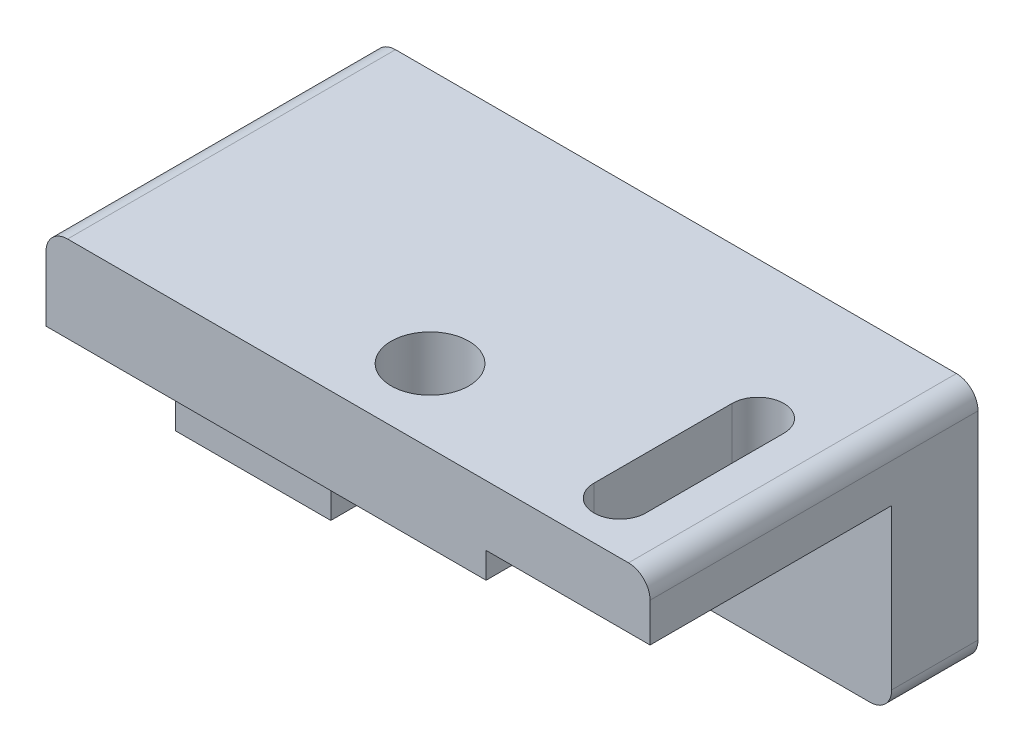
ISO-10303-21;
HEADER;
FILE_DESCRIPTION(('STEP AP214'),'2;1');
FILE_NAME('part.step','',(''),(''),'','','');
FILE_SCHEMA(('AUTOMOTIVE_DESIGN { 1 0 10303 214 1 1 1 1 }'));
ENDSEC;
DATA;
#1=APPLICATION_CONTEXT('core data for automotive mechanical design processes');
#2=APPLICATION_PROTOCOL_DEFINITION('international standard','automotive_design',2000,#1);
#3=PRODUCT_CONTEXT('',#1,'mechanical');
#4=PRODUCT('Part','Part','',(#3));
#5=PRODUCT_RELATED_PRODUCT_CATEGORY('part','',(#4));
#6=PRODUCT_DEFINITION_FORMATION('','',#4);
#7=PRODUCT_DEFINITION_CONTEXT('part definition',#1,'design');
#8=PRODUCT_DEFINITION('design','',#6,#7);
#9=PRODUCT_DEFINITION_SHAPE('','',#8);
#10=(LENGTH_UNIT() NAMED_UNIT(*) SI_UNIT(.MILLI.,.METRE.));
#11=(NAMED_UNIT(*) PLANE_ANGLE_UNIT() SI_UNIT($,.RADIAN.));
#12=(NAMED_UNIT(*) SI_UNIT($,.STERADIAN.) SOLID_ANGLE_UNIT());
#13=UNCERTAINTY_MEASURE_WITH_UNIT(LENGTH_MEASURE(1.E-05),#10,'distance_accuracy_value','');
#14=(GEOMETRIC_REPRESENTATION_CONTEXT(3) GLOBAL_UNCERTAINTY_ASSIGNED_CONTEXT((#13)) GLOBAL_UNIT_ASSIGNED_CONTEXT((#10,
#11,#12)) REPRESENTATION_CONTEXT('',''));
#15=CARTESIAN_POINT('',(0.,0.,0.));
#16=DIRECTION('',(0.,0.,1.));
#17=DIRECTION('',(1.,0.,0.));
#18=AXIS2_PLACEMENT_3D('',#15,#16,#17);
#19=CARTESIAN_POINT('',(0.,-51.,20.));
#20=DIRECTION('',(0.,0.,1.));
#21=DIRECTION('',(0.,-1.,0.));
#22=AXIS2_PLACEMENT_3D('',#19,#20,#21);
#23=PLANE('',#22);
#24=DIRECTION('',(0.,-1.,0.));
#25=VECTOR('',#24,1.);
#26=CARTESIAN_POINT('',(51.,-56.,20.));
#27=LINE('',#26,#25);
#28=CARTESIAN_POINT('',(51.,-34.,20.));
#29=VERTEX_POINT('',#28);
#30=CARTESIAN_POINT('',(51.,-56.,20.));
#31=VERTEX_POINT('',#30);
#32=EDGE_CURVE('E258',#29,#31,#27,.T.);
#33=ORIENTED_EDGE('',*,*,#32,.F.);
#34=DIRECTION('',(-1.,0.,0.));
#35=VECTOR('',#34,1.);
#36=CARTESIAN_POINT('',(51.,-34.,20.));
#37=LINE('',#36,#35);
#38=CARTESIAN_POINT('',(81.,-34.,20.));
#39=VERTEX_POINT('',#38);
#40=EDGE_CURVE('E270',#39,#29,#37,.T.);
#41=ORIENTED_EDGE('',*,*,#40,.F.);
#42=DIRECTION('',(0.,1.,0.));
#43=VECTOR('',#42,1.);
#44=CARTESIAN_POINT('',(81.,-34.,20.));
#45=LINE('',#44,#43);
#46=CARTESIAN_POINT('',(81.,-56.,20.));
#47=VERTEX_POINT('',#46);
#48=EDGE_CURVE('E255',#47,#39,#45,.T.);
#49=ORIENTED_EDGE('',*,*,#48,.F.);
#50=DIRECTION('',(1.,0.,0.));
#51=VECTOR('',#50,1.);
#52=CARTESIAN_POINT('',(36.,-56.,20.));
#53=LINE('',#52,#51);
#54=CARTESIAN_POINT('',(135.,-56.,20.));
#55=VERTEX_POINT('',#54);
#56=EDGE_CURVE('E292',#47,#55,#53,.T.);
#57=ORIENTED_EDGE('',*,*,#56,.T.);
#58=CARTESIAN_POINT('',(135.,-51.,20.));
#59=DIRECTION('',(0.,0.,-1.));
#60=DIRECTION('',(1.,0.,0.));
#61=AXIS2_PLACEMENT_3D('',#58,#59,#60);
#62=CIRCLE('',#61,5.);
#63=CARTESIAN_POINT('',(140.,-51.,20.));
#64=VERTEX_POINT('',#63);
#65=EDGE_CURVE('E283',#64,#55,#62,.T.);
#66=ORIENTED_EDGE('',*,*,#65,.F.);
#67=DIRECTION('',(0.,-1.,0.));
#68=VECTOR('',#67,1.);
#69=CARTESIAN_POINT('',(140.,-51.,20.));
#70=LINE('',#69,#68);
#71=CARTESIAN_POINT('',(140.,-14.,20.));
#72=VERTEX_POINT('',#71);
#73=EDGE_CURVE('E361',#72,#64,#70,.T.);
#74=ORIENTED_EDGE('',*,*,#73,.F.);
#75=DIRECTION('',(-1.,0.,0.));
#76=VECTOR('',#75,1.);
#77=CARTESIAN_POINT('',(140.,-14.,20.));
#78=LINE('',#77,#76);
#79=CARTESIAN_POINT('',(102.,-14.,20.));
#80=VERTEX_POINT('',#79);
#81=EDGE_CURVE('E346',#72,#80,#78,.T.);
#82=ORIENTED_EDGE('',*,*,#81,.T.);
#83=DIRECTION('',(0.,-1.,0.));
#84=VECTOR('',#83,1.);
#85=CARTESIAN_POINT('',(102.,-14.,20.));
#86=LINE('',#85,#84);
#87=CARTESIAN_POINT('',(102.,-20.,20.));
#88=VERTEX_POINT('',#87);
#89=EDGE_CURVE('E352',#80,#88,#86,.T.);
#90=ORIENTED_EDGE('',*,*,#89,.T.);
#91=DIRECTION('',(1.,0.,0.));
#92=VECTOR('',#91,1.);
#93=CARTESIAN_POINT('',(0.,-20.,20.));
#94=LINE('',#93,#92);
#95=CARTESIAN_POINT('',(36.,-20.,20.));
#96=VERTEX_POINT('',#95);
#97=EDGE_CURVE('E369',#96,#88,#94,.T.);
#98=ORIENTED_EDGE('',*,*,#97,.F.);
#99=DIRECTION('',(0.,-1.,0.));
#100=VECTOR('',#99,1.);
#101=CARTESIAN_POINT('',(36.,-20.,20.));
#102=LINE('',#101,#100);
#103=CARTESIAN_POINT('',(36.,-56.,20.));
#104=VERTEX_POINT('',#103);
#105=EDGE_CURVE('E299',#96,#104,#102,.T.);
#106=ORIENTED_EDGE('',*,*,#105,.T.);
#107=EDGE_CURVE('E291',#104,#31,#53,.T.);
#108=ORIENTED_EDGE('',*,*,#107,.T.);
#109=EDGE_LOOP('',(#33,#41,#49,#57,#66,#74,#82,#90,#98,#106,#108));
#110=FACE_BOUND('',#109,.T.);
#111=ADVANCED_FACE('F44',(#110),#23,.T.);
#112=CARTESIAN_POINT('',(140.,-20.,76.));
#113=DIRECTION('',(0.,1.,0.));
#114=DIRECTION('',(0.,0.,1.));
#115=AXIS2_PLACEMENT_3D('',#112,#113,#114);
#116=PLANE('',#115);
#117=CARTESIAN_POINT('',(72.,-20.,59.));
#118=DIRECTION('',(0.,-1.,0.));
#119=DIRECTION('',(0.,0.,-1.));
#120=AXIS2_PLACEMENT_3D('',#117,#118,#119);
#121=CIRCLE('',#120,9.);
#122=CARTESIAN_POINT('',(72.,-20.,50.));
#123=VERTEX_POINT('',#122);
#124=EDGE_CURVE('E276',#123,#123,#121,.T.);
#125=ORIENTED_EDGE('',*,*,#124,.F.);
#126=EDGE_LOOP('',(#125));
#127=FACE_BOUND('',#126,.T.);
#128=DIRECTION('',(0.,0.,-1.));
#129=VECTOR('',#128,1.);
#130=CARTESIAN_POINT('',(0.,-20.,76.));
#131=LINE('',#130,#129);
#132=CARTESIAN_POINT('',(0.,-20.,76.));
#133=VERTEX_POINT('',#132);
#134=CARTESIAN_POINT('',(0.,-20.,46.));
#135=VERTEX_POINT('',#134);
#136=EDGE_CURVE('E388',#133,#135,#131,.T.);
#137=ORIENTED_EDGE('',*,*,#136,.T.);
#138=DIRECTION('',(-1.,0.,0.));
#139=VECTOR('',#138,1.);
#140=CARTESIAN_POINT('',(36.,-20.,46.));
#141=LINE('',#140,#139);
#142=CARTESIAN_POINT('',(36.,-20.,46.));
#143=VERTEX_POINT('',#142);
#144=EDGE_CURVE('E311',#143,#135,#141,.T.);
#145=ORIENTED_EDGE('',*,*,#144,.F.);
#146=DIRECTION('',(0.,0.,-1.));
#147=VECTOR('',#146,1.);
#148=CARTESIAN_POINT('',(36.,-20.,20.));
#149=LINE('',#148,#147);
#150=EDGE_CURVE('E306',#143,#96,#149,.T.);
#151=ORIENTED_EDGE('',*,*,#150,.T.);
#152=ORIENTED_EDGE('',*,*,#97,.T.);
#153=DIRECTION('',(0.,0.,1.));
#154=VECTOR('',#153,1.);
#155=CARTESIAN_POINT('',(102.,-20.,20.));
#156=LINE('',#155,#154);
#157=CARTESIAN_POINT('',(102.,-20.,76.));
#158=VERTEX_POINT('',#157);
#159=EDGE_CURVE('E359',#88,#158,#156,.T.);
#160=ORIENTED_EDGE('',*,*,#159,.T.);
#161=DIRECTION('',(1.,0.,0.));
#162=VECTOR('',#161,1.);
#163=CARTESIAN_POINT('',(140.,-20.,76.));
#164=LINE('',#163,#162);
#165=EDGE_CURVE('E374',#133,#158,#164,.T.);
#166=ORIENTED_EDGE('',*,*,#165,.F.);
#167=EDGE_LOOP('',(#137,#145,#151,#152,#160,#166));
#168=FACE_BOUND('',#167,.T.);
#169=ADVANCED_FACE('F50',(#127,#168),#116,.F.);
#170=CARTESIAN_POINT('',(140.,-5.00000000000004,76.));
#171=DIRECTION('',(-1.,0.,0.));
#172=DIRECTION('',(0.,0.,1.));
#173=AXIS2_PLACEMENT_3D('',#170,#171,#172);
#174=PLANE('',#173);
#175=ORIENTED_EDGE('',*,*,#73,.T.);
#176=DIRECTION('',(0.,0.,1.));
#177=VECTOR('',#176,1.);
#178=CARTESIAN_POINT('',(140.,-51.,-84.));
#179=LINE('',#178,#177);
#180=CARTESIAN_POINT('',(140.,-51.,0.));
#181=VERTEX_POINT('',#180);
#182=EDGE_CURVE('E289',#181,#64,#179,.T.);
#183=ORIENTED_EDGE('',*,*,#182,.F.);
#184=DIRECTION('',(0.,1.,0.));
#185=VECTOR('',#184,1.);
#186=CARTESIAN_POINT('',(140.,-5.00000000000004,0.));
#187=LINE('',#186,#185);
#188=CARTESIAN_POINT('',(140.,-5.00000000000004,0.));
#189=VERTEX_POINT('',#188);
#190=EDGE_CURVE('E372',#181,#189,#187,.T.);
#191=ORIENTED_EDGE('',*,*,#190,.T.);
#192=DIRECTION('',(0.,0.,-1.));
#193=VECTOR('',#192,1.);
#194=CARTESIAN_POINT('',(140.,-5.00000000000004,76.));
#195=LINE('',#194,#193);
#196=CARTESIAN_POINT('',(140.,-5.00000000000004,76.));
#197=VERTEX_POINT('',#196);
#198=EDGE_CURVE('E53',#197,#189,#195,.T.);
#199=ORIENTED_EDGE('',*,*,#198,.F.);
#200=DIRECTION('',(0.,1.,0.));
#201=VECTOR('',#200,1.);
#202=CARTESIAN_POINT('',(140.,-5.00000000000004,76.));
#203=LINE('',#202,#201);
#204=CARTESIAN_POINT('',(140.,-14.,76.));
#205=VERTEX_POINT('',#204);
#206=EDGE_CURVE('E377',#205,#197,#203,.T.);
#207=ORIENTED_EDGE('',*,*,#206,.F.);
#208=DIRECTION('',(0.,0.,1.));
#209=VECTOR('',#208,1.);
#210=CARTESIAN_POINT('',(140.,-14.,20.));
#211=LINE('',#210,#209);
#212=EDGE_CURVE('E358',#72,#205,#211,.T.);
#213=ORIENTED_EDGE('',*,*,#212,.F.);
#214=EDGE_LOOP('',(#175,#183,#191,#199,#207,#213));
#215=FACE_BOUND('',#214,.T.);
#216=ADVANCED_FACE('F439',(#215),#174,.F.);
#217=CARTESIAN_POINT('',(135.,-5.,76.));
#218=DIRECTION('',(0.,0.,-1.));
#219=DIRECTION('',(-1.,0.,0.));
#220=AXIS2_PLACEMENT_3D('',#217,#218,#219);
#221=CYLINDRICAL_SURFACE('',#220,5.);
#222=CARTESIAN_POINT('',(135.,-5.,0.));
#223=DIRECTION('',(0.,0.,1.));
#224=DIRECTION('',(1.,0.,0.));
#225=AXIS2_PLACEMENT_3D('',#222,#223,#224);
#226=CIRCLE('',#225,5.);
#227=CARTESIAN_POINT('',(135.,0.,0.));
#228=VERTEX_POINT('',#227);
#229=EDGE_CURVE('E392',#189,#228,#226,.T.);
#230=ORIENTED_EDGE('',*,*,#229,.T.);
#231=DIRECTION('',(0.,0.,-1.));
#232=VECTOR('',#231,1.);
#233=CARTESIAN_POINT('',(135.,0.,76.));
#234=LINE('',#233,#232);
#235=CARTESIAN_POINT('',(135.,0.,76.));
#236=VERTEX_POINT('',#235);
#237=EDGE_CURVE('E409',#236,#228,#234,.T.);
#238=ORIENTED_EDGE('',*,*,#237,.F.);
#239=CARTESIAN_POINT('',(135.,-5.,76.));
#240=DIRECTION('',(0.,0.,1.));
#241=DIRECTION('',(1.,0.,0.));
#242=AXIS2_PLACEMENT_3D('',#239,#240,#241);
#243=CIRCLE('',#242,5.);
#244=EDGE_CURVE('E382',#197,#236,#243,.T.);
#245=ORIENTED_EDGE('',*,*,#244,.F.);
#246=ORIENTED_EDGE('',*,*,#198,.T.);
#247=EDGE_LOOP('',(#230,#238,#245,#246));
#248=FACE_BOUND('',#247,.T.);
#249=ADVANCED_FACE('F411',(#248),#221,.T.);
#250=CARTESIAN_POINT('',(5.00000000000004,0.,76.));
#251=DIRECTION('',(0.,-1.,0.));
#252=DIRECTION('',(0.,0.,-1.));
#253=AXIS2_PLACEMENT_3D('',#250,#251,#252);
#254=PLANE('',#253);
#255=CARTESIAN_POINT('',(72.,0.,59.));
#256=DIRECTION('',(0.,-1.,0.));
#257=DIRECTION('',(0.,0.,-1.));
#258=AXIS2_PLACEMENT_3D('',#255,#256,#257);
#259=CIRCLE('',#258,9.);
#260=CARTESIAN_POINT('',(72.,0.,50.));
#261=VERTEX_POINT('',#260);
#262=EDGE_CURVE('E47',#261,#261,#259,.T.);
#263=ORIENTED_EDGE('',*,*,#262,.T.);
#264=EDGE_LOOP('',(#263));
#265=FACE_BOUND('',#264,.T.);
#266=DIRECTION('',(0.,0.,1.));
#267=VECTOR('',#266,1.);
#268=CARTESIAN_POINT('',(127.,0.,76.));
#269=LINE('',#268,#267);
#270=CARTESIAN_POINT('',(127.,0.,32.));
#271=VERTEX_POINT('',#270);
#272=CARTESIAN_POINT('',(127.,0.,64.));
#273=VERTEX_POINT('',#272);
#274=EDGE_CURVE('E341',#271,#273,#269,.T.);
#275=ORIENTED_EDGE('',*,*,#274,.T.);
#276=CARTESIAN_POINT('',(121.,0.,64.));
#277=DIRECTION('',(0.,-1.,0.));
#278=DIRECTION('',(0.,0.,-1.));
#279=AXIS2_PLACEMENT_3D('',#276,#277,#278);
#280=CIRCLE('',#279,6.);
#281=CARTESIAN_POINT('',(115.,0.,64.));
#282=VERTEX_POINT('',#281);
#283=EDGE_CURVE('E342',#273,#282,#280,.T.);
#284=ORIENTED_EDGE('',*,*,#283,.T.);
#285=DIRECTION('',(0.,0.,-1.));
#286=VECTOR('',#285,1.);
#287=CARTESIAN_POINT('',(115.,0.,76.));
#288=LINE('',#287,#286);
#289=CARTESIAN_POINT('',(115.,0.,32.));
#290=VERTEX_POINT('',#289);
#291=EDGE_CURVE('E328',#282,#290,#288,.T.);
#292=ORIENTED_EDGE('',*,*,#291,.T.);
#293=CARTESIAN_POINT('',(121.,0.,32.));
#294=DIRECTION('',(0.,-1.,0.));
#295=DIRECTION('',(0.,0.,-1.));
#296=AXIS2_PLACEMENT_3D('',#293,#294,#295);
#297=CIRCLE('',#296,6.);
#298=EDGE_CURVE('E339',#290,#271,#297,.T.);
#299=ORIENTED_EDGE('',*,*,#298,.T.);
#300=EDGE_LOOP('',(#275,#284,#292,#299));
#301=FACE_BOUND('',#300,.T.);
#302=DIRECTION('',(-1.,0.,0.));
#303=VECTOR('',#302,1.);
#304=CARTESIAN_POINT('',(5.00000000000004,0.,0.));
#305=LINE('',#304,#303);
#306=CARTESIAN_POINT('',(5.00000000000004,0.,0.));
#307=VERTEX_POINT('',#306);
#308=EDGE_CURVE('E395',#228,#307,#305,.T.);
#309=ORIENTED_EDGE('',*,*,#308,.T.);
#310=DIRECTION('',(0.,0.,-1.));
#311=VECTOR('',#310,1.);
#312=CARTESIAN_POINT('',(5.00000000000004,0.,76.));
#313=LINE('',#312,#311);
#314=CARTESIAN_POINT('',(5.00000000000004,0.,76.));
#315=VERTEX_POINT('',#314);
#316=EDGE_CURVE('E401',#315,#307,#313,.T.);
#317=ORIENTED_EDGE('',*,*,#316,.F.);
#318=DIRECTION('',(-1.,0.,0.));
#319=VECTOR('',#318,1.);
#320=CARTESIAN_POINT('',(5.00000000000004,0.,76.));
#321=LINE('',#320,#319);
#322=EDGE_CURVE('E384',#236,#315,#321,.T.);
#323=ORIENTED_EDGE('',*,*,#322,.F.);
#324=ORIENTED_EDGE('',*,*,#237,.T.);
#325=EDGE_LOOP('',(#309,#317,#323,#324));
#326=FACE_BOUND('',#325,.T.);
#327=ADVANCED_FACE('F430',(#265,#301,#326),#254,.F.);
#328=CARTESIAN_POINT('',(5.,-5.,76.));
#329=DIRECTION('',(0.,0.,-1.));
#330=DIRECTION('',(-1.,0.,0.));
#331=AXIS2_PLACEMENT_3D('',#328,#329,#330);
#332=CYLINDRICAL_SURFACE('',#331,5.);
#333=CARTESIAN_POINT('',(5.,-5.,0.));
#334=DIRECTION('',(0.,0.,1.));
#335=DIRECTION('',(-1.,0.,0.));
#336=AXIS2_PLACEMENT_3D('',#333,#334,#335);
#337=CIRCLE('',#336,5.);
#338=CARTESIAN_POINT('',(0.,-5.00000000000003,0.));
#339=VERTEX_POINT('',#338);
#340=EDGE_CURVE('E393',#307,#339,#337,.T.);
#341=ORIENTED_EDGE('',*,*,#340,.T.);
#342=DIRECTION('',(0.,0.,-1.));
#343=VECTOR('',#342,1.);
#344=CARTESIAN_POINT('',(0.,-5.00000000000003,76.));
#345=LINE('',#344,#343);
#346=CARTESIAN_POINT('',(0.,-5.00000000000003,76.));
#347=VERTEX_POINT('',#346);
#348=EDGE_CURVE('E400',#347,#339,#345,.T.);
#349=ORIENTED_EDGE('',*,*,#348,.F.);
#350=CARTESIAN_POINT('',(5.,-5.,76.));
#351=DIRECTION('',(0.,0.,1.));
#352=DIRECTION('',(-1.,0.,0.));
#353=AXIS2_PLACEMENT_3D('',#350,#351,#352);
#354=CIRCLE('',#353,5.);
#355=EDGE_CURVE('E383',#315,#347,#354,.T.);
#356=ORIENTED_EDGE('',*,*,#355,.F.);
#357=ORIENTED_EDGE('',*,*,#316,.T.);
#358=EDGE_LOOP('',(#341,#349,#356,#357));
#359=FACE_BOUND('',#358,.T.);
#360=ADVANCED_FACE('F431',(#359),#332,.T.);
#361=CARTESIAN_POINT('',(0.,-20.,76.));
#362=DIRECTION('',(1.,0.,0.));
#363=DIRECTION('',(0.,0.,-1.));
#364=AXIS2_PLACEMENT_3D('',#361,#362,#363);
#365=PLANE('',#364);
#366=DIRECTION('',(0.,1.,0.));
#367=VECTOR('',#366,1.);
#368=CARTESIAN_POINT('',(0.,-29.5,27.));
#369=LINE('',#368,#367);
#370=CARTESIAN_POINT('',(0.,-46.5,27.));
#371=VERTEX_POINT('',#370);
#372=CARTESIAN_POINT('',(0.,-29.5,27.));
#373=VERTEX_POINT('',#372);
#374=EDGE_CURVE('E218',#371,#373,#369,.T.);
#375=ORIENTED_EDGE('',*,*,#374,.T.);
#376=CARTESIAN_POINT('',(0.,-29.5,33.));
#377=DIRECTION('',(1.,0.,0.));
#378=DIRECTION('',(0.,0.,-1.));
#379=AXIS2_PLACEMENT_3D('',#376,#377,#378);
#380=CIRCLE('',#379,6.);
#381=CARTESIAN_POINT('',(0.,-29.5,39.));
#382=VERTEX_POINT('',#381);
#383=EDGE_CURVE('E213',#373,#382,#380,.T.);
#384=ORIENTED_EDGE('',*,*,#383,.T.);
#385=DIRECTION('',(0.,-1.,0.));
#386=VECTOR('',#385,1.);
#387=CARTESIAN_POINT('',(0.,-29.5,39.));
#388=LINE('',#387,#386);
#389=CARTESIAN_POINT('',(0.,-46.5,39.));
#390=VERTEX_POINT('',#389);
#391=EDGE_CURVE('E224',#382,#390,#388,.T.);
#392=ORIENTED_EDGE('',*,*,#391,.T.);
#393=CARTESIAN_POINT('',(0.,-46.5,33.));
#394=DIRECTION('',(1.,0.,0.));
#395=DIRECTION('',(0.,0.,-1.));
#396=AXIS2_PLACEMENT_3D('',#393,#394,#395);
#397=CIRCLE('',#396,6.00000000000001);
#398=EDGE_CURVE('E64',#390,#371,#397,.T.);
#399=ORIENTED_EDGE('',*,*,#398,.T.);
#400=EDGE_LOOP('',(#375,#384,#392,#399));
#401=FACE_BOUND('',#400,.T.);
#402=DIRECTION('',(0.,0.,-1.));
#403=VECTOR('',#402,1.);
#404=CARTESIAN_POINT('',(0.,-56.,5.00000000000004));
#405=LINE('',#404,#403);
#406=CARTESIAN_POINT('',(0.,-56.,46.));
#407=VERTEX_POINT('',#406);
#408=CARTESIAN_POINT('',(0.,-56.,0.));
#409=VERTEX_POINT('',#408);
#410=EDGE_CURVE('E370',#407,#409,#405,.T.);
#411=ORIENTED_EDGE('',*,*,#410,.F.);
#412=DIRECTION('',(0.,1.,0.));
#413=VECTOR('',#412,1.);
#414=CARTESIAN_POINT('',(0.,-20.,46.));
#415=LINE('',#414,#413);
#416=EDGE_CURVE('E296',#407,#135,#415,.T.);
#417=ORIENTED_EDGE('',*,*,#416,.T.);
#418=ORIENTED_EDGE('',*,*,#136,.F.);
#419=DIRECTION('',(0.,-1.,0.));
#420=VECTOR('',#419,1.);
#421=CARTESIAN_POINT('',(0.,-20.,76.));
#422=LINE('',#421,#420);
#423=EDGE_CURVE('E386',#347,#133,#422,.T.);
#424=ORIENTED_EDGE('',*,*,#423,.F.);
#425=ORIENTED_EDGE('',*,*,#348,.T.);
#426=DIRECTION('',(0.,-1.,0.));
#427=VECTOR('',#426,1.);
#428=CARTESIAN_POINT('',(0.,-20.,0.));
#429=LINE('',#428,#427);
#430=EDGE_CURVE('E378',#339,#409,#429,.T.);
#431=ORIENTED_EDGE('',*,*,#430,.T.);
#432=EDGE_LOOP('',(#411,#417,#418,#424,#425,#431));
#433=FACE_BOUND('',#432,.T.);
#434=ADVANCED_FACE('F227',(#401,#433),#365,.F.);
#435=CARTESIAN_POINT('',(5.,-5.,76.));
#436=DIRECTION('',(0.,0.,-1.));
#437=DIRECTION('',(-1.,0.,0.));
#438=AXIS2_PLACEMENT_3D('',#435,#436,#437);
#439=PLANE('',#438);
#440=ORIENTED_EDGE('',*,*,#165,.T.);
#441=DIRECTION('',(0.,-1.,0.));
#442=VECTOR('',#441,1.);
#443=CARTESIAN_POINT('',(102.,-14.,76.));
#444=LINE('',#443,#442);
#445=CARTESIAN_POINT('',(102.,-14.,76.));
#446=VERTEX_POINT('',#445);
#447=EDGE_CURVE('E354',#446,#158,#444,.T.);
#448=ORIENTED_EDGE('',*,*,#447,.F.);
#449=DIRECTION('',(-1.,0.,0.));
#450=VECTOR('',#449,1.);
#451=CARTESIAN_POINT('',(140.,-14.,76.));
#452=LINE('',#451,#450);
#453=EDGE_CURVE('E350',#205,#446,#452,.T.);
#454=ORIENTED_EDGE('',*,*,#453,.F.);
#455=ORIENTED_EDGE('',*,*,#206,.T.);
#456=ORIENTED_EDGE('',*,*,#244,.T.);
#457=ORIENTED_EDGE('',*,*,#322,.T.);
#458=ORIENTED_EDGE('',*,*,#355,.T.);
#459=ORIENTED_EDGE('',*,*,#423,.T.);
#460=EDGE_LOOP('',(#440,#448,#454,#455,#456,#457,#458,#459));
#461=FACE_BOUND('',#460,.T.);
#462=ADVANCED_FACE('F434',(#461),#439,.F.);
#463=CARTESIAN_POINT('',(5.,-5.,0.));
#464=DIRECTION('',(0.,0.,-1.));
#465=DIRECTION('',(-1.,0.,0.));
#466=AXIS2_PLACEMENT_3D('',#463,#464,#465);
#467=PLANE('',#466);
#468=CARTESIAN_POINT('',(66.,-45.,0.));
#469=DIRECTION('',(0.,0.,1.));
#470=DIRECTION('',(1.,0.,0.));
#471=AXIS2_PLACEMENT_3D('',#468,#469,#470);
#472=CIRCLE('',#471,6.);
#473=CARTESIAN_POINT('',(72.,-45.,0.));
#474=VERTEX_POINT('',#473);
#475=EDGE_CURVE('E248',#474,#474,#472,.T.);
#476=ORIENTED_EDGE('',*,*,#475,.T.);
#477=EDGE_LOOP('',(#476));
#478=FACE_BOUND('',#477,.T.);
#479=CARTESIAN_POINT('',(135.,-51.,0.));
#480=DIRECTION('',(0.,0.,-1.));
#481=DIRECTION('',(-1.,0.,0.));
#482=AXIS2_PLACEMENT_3D('',#479,#480,#481);
#483=CIRCLE('',#482,5.);
#484=CARTESIAN_POINT('',(135.,-56.,0.));
#485=VERTEX_POINT('',#484);
#486=EDGE_CURVE('E290',#485,#181,#483,.F.);
#487=ORIENTED_EDGE('',*,*,#486,.F.);
#488=DIRECTION('',(-1.,0.,0.));
#489=VECTOR('',#488,1.);
#490=CARTESIAN_POINT('',(140.,-56.,0.));
#491=LINE('',#490,#489);
#492=EDGE_CURVE('E298',#485,#409,#491,.T.);
#493=ORIENTED_EDGE('',*,*,#492,.T.);
#494=ORIENTED_EDGE('',*,*,#430,.F.);
#495=ORIENTED_EDGE('',*,*,#340,.F.);
#496=ORIENTED_EDGE('',*,*,#308,.F.);
#497=ORIENTED_EDGE('',*,*,#229,.F.);
#498=ORIENTED_EDGE('',*,*,#190,.F.);
#499=EDGE_LOOP('',(#487,#493,#494,#495,#496,#497,#498));
#500=FACE_BOUND('',#499,.T.);
#501=ADVANCED_FACE('F422',(#478,#500),#467,.T.);
#502=CARTESIAN_POINT('',(0.,-56.,5.00000000000004));
#503=DIRECTION('',(0.,-1.,0.));
#504=DIRECTION('',(0.,0.,-1.));
#505=AXIS2_PLACEMENT_3D('',#502,#503,#504);
#506=PLANE('',#505);
#507=DIRECTION('',(0.,0.,1.));
#508=VECTOR('',#507,1.);
#509=CARTESIAN_POINT('',(51.,-56.,10.));
#510=LINE('',#509,#508);
#511=CARTESIAN_POINT('',(51.,-56.,10.));
#512=VERTEX_POINT('',#511);
#513=EDGE_CURVE('E274',#512,#31,#510,.T.);
#514=ORIENTED_EDGE('',*,*,#513,.T.);
#515=ORIENTED_EDGE('',*,*,#107,.F.);
#516=DIRECTION('',(0.,0.,1.));
#517=VECTOR('',#516,1.);
#518=CARTESIAN_POINT('',(36.,-56.,46.));
#519=LINE('',#518,#517);
#520=CARTESIAN_POINT('',(36.,-56.,46.));
#521=VERTEX_POINT('',#520);
#522=EDGE_CURVE('E301',#104,#521,#519,.T.);
#523=ORIENTED_EDGE('',*,*,#522,.T.);
#524=DIRECTION('',(-1.,0.,0.));
#525=VECTOR('',#524,1.);
#526=CARTESIAN_POINT('',(36.,-56.,46.));
#527=LINE('',#526,#525);
#528=EDGE_CURVE('E308',#521,#407,#527,.T.);
#529=ORIENTED_EDGE('',*,*,#528,.T.);
#530=ORIENTED_EDGE('',*,*,#410,.T.);
#531=ORIENTED_EDGE('',*,*,#492,.F.);
#532=DIRECTION('',(0.,0.,1.));
#533=VECTOR('',#532,1.);
#534=CARTESIAN_POINT('',(135.,-56.,-84.));
#535=LINE('',#534,#533);
#536=EDGE_CURVE('E11',#55,#485,#535,.F.);
#537=ORIENTED_EDGE('',*,*,#536,.F.);
#538=ORIENTED_EDGE('',*,*,#56,.F.);
#539=DIRECTION('',(0.,0.,1.));
#540=VECTOR('',#539,1.);
#541=CARTESIAN_POINT('',(81.,-56.,10.));
#542=LINE('',#541,#540);
#543=CARTESIAN_POINT('',(81.,-56.,10.));
#544=VERTEX_POINT('',#543);
#545=EDGE_CURVE('E267',#544,#47,#542,.T.);
#546=ORIENTED_EDGE('',*,*,#545,.F.);
#547=DIRECTION('',(1.,0.,0.));
#548=VECTOR('',#547,1.);
#549=CARTESIAN_POINT('',(81.,-56.,10.));
#550=LINE('',#549,#548);
#551=EDGE_CURVE('E253',#512,#544,#550,.T.);
#552=ORIENTED_EDGE('',*,*,#551,.F.);
#553=EDGE_LOOP('',(#514,#515,#523,#529,#530,#531,#537,#538,#546,#552));
#554=FACE_BOUND('',#553,.T.);
#555=ADVANCED_FACE('F463',(#554),#506,.T.);
#556=CARTESIAN_POINT('',(102.,-14.,20.));
#557=DIRECTION('',(-1.,0.,0.));
#558=DIRECTION('',(0.,0.,1.));
#559=AXIS2_PLACEMENT_3D('',#556,#557,#558);
#560=PLANE('',#559);
#561=ORIENTED_EDGE('',*,*,#447,.T.);
#562=ORIENTED_EDGE('',*,*,#159,.F.);
#563=ORIENTED_EDGE('',*,*,#89,.F.);
#564=DIRECTION('',(0.,0.,1.));
#565=VECTOR('',#564,1.);
#566=CARTESIAN_POINT('',(102.,-14.,20.));
#567=LINE('',#566,#565);
#568=EDGE_CURVE('E364',#80,#446,#567,.T.);
#569=ORIENTED_EDGE('',*,*,#568,.T.);
#570=EDGE_LOOP('',(#561,#562,#563,#569));
#571=FACE_BOUND('',#570,.T.);
#572=ADVANCED_FACE('F451',(#571),#560,.F.);
#573=CARTESIAN_POINT('',(140.,-14.,20.));
#574=DIRECTION('',(0.,1.,0.));
#575=DIRECTION('',(0.,0.,1.));
#576=AXIS2_PLACEMENT_3D('',#573,#574,#575);
#577=PLANE('',#576);
#578=DIRECTION('',(0.,0.,-1.));
#579=VECTOR('',#578,1.);
#580=CARTESIAN_POINT('',(115.,-14.,64.));
#581=LINE('',#580,#579);
#582=CARTESIAN_POINT('',(115.,-14.,64.));
#583=VERTEX_POINT('',#582);
#584=CARTESIAN_POINT('',(115.,-14.,32.));
#585=VERTEX_POINT('',#584);
#586=EDGE_CURVE('E319',#583,#585,#581,.T.);
#587=ORIENTED_EDGE('',*,*,#586,.F.);
#588=CARTESIAN_POINT('',(121.,-14.,64.));
#589=DIRECTION('',(0.,-1.,0.));
#590=DIRECTION('',(0.,0.,-1.));
#591=AXIS2_PLACEMENT_3D('',#588,#589,#590);
#592=CIRCLE('',#591,6.);
#593=CARTESIAN_POINT('',(127.,-14.,64.));
#594=VERTEX_POINT('',#593);
#595=EDGE_CURVE('E313',#594,#583,#592,.T.);
#596=ORIENTED_EDGE('',*,*,#595,.F.);
#597=DIRECTION('',(0.,0.,1.));
#598=VECTOR('',#597,1.);
#599=CARTESIAN_POINT('',(127.,-14.,64.));
#600=LINE('',#599,#598);
#601=CARTESIAN_POINT('',(127.,-14.,32.));
#602=VERTEX_POINT('',#601);
#603=EDGE_CURVE('E323',#602,#594,#600,.T.);
#604=ORIENTED_EDGE('',*,*,#603,.F.);
#605=CARTESIAN_POINT('',(121.,-14.,32.));
#606=DIRECTION('',(0.,-1.,0.));
#607=DIRECTION('',(0.,0.,-1.));
#608=AXIS2_PLACEMENT_3D('',#605,#606,#607);
#609=CIRCLE('',#608,6.);
#610=EDGE_CURVE('E324',#585,#602,#609,.T.);
#611=ORIENTED_EDGE('',*,*,#610,.F.);
#612=EDGE_LOOP('',(#587,#596,#604,#611));
#613=FACE_BOUND('',#612,.T.);
#614=ORIENTED_EDGE('',*,*,#453,.T.);
#615=ORIENTED_EDGE('',*,*,#568,.F.);
#616=ORIENTED_EDGE('',*,*,#81,.F.);
#617=ORIENTED_EDGE('',*,*,#212,.T.);
#618=EDGE_LOOP('',(#614,#615,#616,#617));
#619=FACE_BOUND('',#618,.T.);
#620=ADVANCED_FACE('F443',(#613,#619),#577,.F.);
#621=CARTESIAN_POINT('',(121.,42.,64.));
#622=DIRECTION('',(0.,-1.,0.));
#623=DIRECTION('',(0.,0.,-1.));
#624=AXIS2_PLACEMENT_3D('',#621,#622,#623);
#625=CYLINDRICAL_SURFACE('',#624,6.);
#626=DIRECTION('',(0.,-1.,0.));
#627=VECTOR('',#626,1.);
#628=CARTESIAN_POINT('',(127.,42.,64.));
#629=LINE('',#628,#627);
#630=EDGE_CURVE('E330',#273,#594,#629,.T.);
#631=ORIENTED_EDGE('',*,*,#630,.T.);
#632=ORIENTED_EDGE('',*,*,#595,.T.);
#633=DIRECTION('',(0.,-1.,0.));
#634=VECTOR('',#633,1.);
#635=CARTESIAN_POINT('',(115.,42.,64.));
#636=LINE('',#635,#634);
#637=EDGE_CURVE('E329',#282,#583,#636,.T.);
#638=ORIENTED_EDGE('',*,*,#637,.F.);
#639=ORIENTED_EDGE('',*,*,#283,.F.);
#640=EDGE_LOOP('',(#631,#632,#638,#639));
#641=FACE_BOUND('',#640,.T.);
#642=ADVANCED_FACE('F555',(#641),#625,.F.);
#643=CARTESIAN_POINT('',(127.,42.,64.));
#644=DIRECTION('',(1.,0.,0.));
#645=DIRECTION('',(0.,0.,-1.));
#646=AXIS2_PLACEMENT_3D('',#643,#644,#645);
#647=PLANE('',#646);
#648=DIRECTION('',(0.,-1.,0.));
#649=VECTOR('',#648,1.);
#650=CARTESIAN_POINT('',(127.,42.,32.));
#651=LINE('',#650,#649);
#652=EDGE_CURVE('E331',#271,#602,#651,.T.);
#653=ORIENTED_EDGE('',*,*,#652,.T.);
#654=ORIENTED_EDGE('',*,*,#603,.T.);
#655=ORIENTED_EDGE('',*,*,#630,.F.);
#656=ORIENTED_EDGE('',*,*,#274,.F.);
#657=EDGE_LOOP('',(#653,#654,#655,#656));
#658=FACE_BOUND('',#657,.T.);
#659=ADVANCED_FACE('F560',(#658),#647,.F.);
#660=CARTESIAN_POINT('',(121.,42.,32.));
#661=DIRECTION('',(0.,-1.,0.));
#662=DIRECTION('',(0.,0.,-1.));
#663=AXIS2_PLACEMENT_3D('',#660,#661,#662);
#664=CYLINDRICAL_SURFACE('',#663,6.);
#665=DIRECTION('',(0.,-1.,0.));
#666=VECTOR('',#665,1.);
#667=CARTESIAN_POINT('',(115.,42.,32.));
#668=LINE('',#667,#666);
#669=EDGE_CURVE('E334',#290,#585,#668,.T.);
#670=ORIENTED_EDGE('',*,*,#669,.T.);
#671=ORIENTED_EDGE('',*,*,#610,.T.);
#672=ORIENTED_EDGE('',*,*,#652,.F.);
#673=ORIENTED_EDGE('',*,*,#298,.F.);
#674=EDGE_LOOP('',(#670,#671,#672,#673));
#675=FACE_BOUND('',#674,.T.);
#676=ADVANCED_FACE('F564',(#675),#664,.F.);
#677=CARTESIAN_POINT('',(115.,42.,64.));
#678=DIRECTION('',(-1.,0.,0.));
#679=DIRECTION('',(0.,0.,1.));
#680=AXIS2_PLACEMENT_3D('',#677,#678,#679);
#681=PLANE('',#680);
#682=ORIENTED_EDGE('',*,*,#637,.T.);
#683=ORIENTED_EDGE('',*,*,#586,.T.);
#684=ORIENTED_EDGE('',*,*,#669,.F.);
#685=ORIENTED_EDGE('',*,*,#291,.F.);
#686=EDGE_LOOP('',(#682,#683,#684,#685));
#687=FACE_BOUND('',#686,.T.);
#688=ADVANCED_FACE('F572',(#687),#681,.F.);
#689=CARTESIAN_POINT('',(36.,-20.,46.));
#690=DIRECTION('',(0.,0.,1.));
#691=DIRECTION('',(1.,0.,0.));
#692=AXIS2_PLACEMENT_3D('',#689,#690,#691);
#693=PLANE('',#692);
#694=ORIENTED_EDGE('',*,*,#416,.F.);
#695=ORIENTED_EDGE('',*,*,#528,.F.);
#696=DIRECTION('',(0.,1.,0.));
#697=VECTOR('',#696,1.);
#698=CARTESIAN_POINT('',(36.,-20.,46.));
#699=LINE('',#698,#697);
#700=EDGE_CURVE('E303',#521,#143,#699,.T.);
#701=ORIENTED_EDGE('',*,*,#700,.T.);
#702=ORIENTED_EDGE('',*,*,#144,.T.);
#703=EDGE_LOOP('',(#694,#695,#701,#702));
#704=FACE_BOUND('',#703,.T.);
#705=ADVANCED_FACE('F470',(#704),#693,.T.);
#706=CARTESIAN_POINT('',(36.,-51.,15.));
#707=DIRECTION('',(-1.,0.,0.));
#708=DIRECTION('',(0.,0.,1.));
#709=AXIS2_PLACEMENT_3D('',#706,#707,#708);
#710=PLANE('',#709);
#711=DIRECTION('',(0.,-1.,0.));
#712=VECTOR('',#711,1.);
#713=CARTESIAN_POINT('',(36.,-29.5,39.));
#714=LINE('',#713,#712);
#715=CARTESIAN_POINT('',(36.,-29.5,39.));
#716=VERTEX_POINT('',#715);
#717=CARTESIAN_POINT('',(36.,-46.5,39.));
#718=VERTEX_POINT('',#717);
#719=EDGE_CURVE('E237',#716,#718,#714,.T.);
#720=ORIENTED_EDGE('',*,*,#719,.F.);
#721=CARTESIAN_POINT('',(36.,-29.5,33.));
#722=DIRECTION('',(1.,0.,0.));
#723=DIRECTION('',(0.,0.,-1.));
#724=AXIS2_PLACEMENT_3D('',#721,#722,#723);
#725=CIRCLE('',#724,6.);
#726=CARTESIAN_POINT('',(36.,-29.5,27.));
#727=VERTEX_POINT('',#726);
#728=EDGE_CURVE('E66',#727,#716,#725,.T.);
#729=ORIENTED_EDGE('',*,*,#728,.F.);
#730=DIRECTION('',(0.,1.,0.));
#731=VECTOR('',#730,1.);
#732=CARTESIAN_POINT('',(36.,-29.5,27.));
#733=LINE('',#732,#731);
#734=CARTESIAN_POINT('',(36.,-46.5,27.));
#735=VERTEX_POINT('',#734);
#736=EDGE_CURVE('E229',#735,#727,#733,.T.);
#737=ORIENTED_EDGE('',*,*,#736,.F.);
#738=CARTESIAN_POINT('',(36.,-46.5,33.));
#739=DIRECTION('',(1.,0.,0.));
#740=DIRECTION('',(0.,0.,-1.));
#741=AXIS2_PLACEMENT_3D('',#738,#739,#740);
#742=CIRCLE('',#741,6.00000000000001);
#743=EDGE_CURVE('E231',#718,#735,#742,.T.);
#744=ORIENTED_EDGE('',*,*,#743,.F.);
#745=EDGE_LOOP('',(#720,#729,#737,#744));
#746=FACE_BOUND('',#745,.T.);
#747=ORIENTED_EDGE('',*,*,#522,.F.);
#748=ORIENTED_EDGE('',*,*,#105,.F.);
#749=ORIENTED_EDGE('',*,*,#150,.F.);
#750=ORIENTED_EDGE('',*,*,#700,.F.);
#751=EDGE_LOOP('',(#747,#748,#749,#750));
#752=FACE_BOUND('',#751,.T.);
#753=ADVANCED_FACE('F458',(#746,#752),#710,.F.);
#754=CARTESIAN_POINT('',(135.,-51.,-84.));
#755=DIRECTION('',(0.,0.,1.));
#756=DIRECTION('',(1.,0.,0.));
#757=AXIS2_PLACEMENT_3D('',#754,#755,#756);
#758=CYLINDRICAL_SURFACE('',#757,5.);
#759=ORIENTED_EDGE('',*,*,#486,.T.);
#760=ORIENTED_EDGE('',*,*,#182,.T.);
#761=ORIENTED_EDGE('',*,*,#65,.T.);
#762=ORIENTED_EDGE('',*,*,#536,.T.);
#763=EDGE_LOOP('',(#759,#760,#761,#762));
#764=FACE_BOUND('',#763,.T.);
#765=ADVANCED_FACE('F471',(#764),#758,.T.);
#766=CARTESIAN_POINT('',(72.,84.,59.));
#767=DIRECTION('',(0.,-1.,0.));
#768=DIRECTION('',(0.,0.,-1.));
#769=AXIS2_PLACEMENT_3D('',#766,#767,#768);
#770=CYLINDRICAL_SURFACE('',#769,9.);
#771=CARTESIAN_POINT('',(72.,-20.,50.));
#772=CARTESIAN_POINT('',(72.,-19.7916666666667,50.));
#773=CARTESIAN_POINT('',(72.,-19.5833333333333,50.));
#774=CARTESIAN_POINT('',(72.,-19.1666666666667,50.));
#775=CARTESIAN_POINT('',(72.,-18.9583333333333,50.));
#776=CARTESIAN_POINT('',(72.,-18.5416666666667,50.));
#777=CARTESIAN_POINT('',(72.,-18.3333333333333,50.));
#778=CARTESIAN_POINT('',(72.,-17.9166666666667,50.));
#779=CARTESIAN_POINT('',(72.,-17.7083333333333,50.));
#780=CARTESIAN_POINT('',(72.,-17.2916666666667,50.));
#781=CARTESIAN_POINT('',(72.,-17.0833333333333,50.));
#782=CARTESIAN_POINT('',(72.,-16.6666666666667,50.));
#783=CARTESIAN_POINT('',(72.,-16.4583333333333,50.));
#784=CARTESIAN_POINT('',(72.,-16.0416666666667,50.));
#785=CARTESIAN_POINT('',(72.,-15.8333333333333,50.));
#786=CARTESIAN_POINT('',(72.,-15.4166666666667,50.));
#787=CARTESIAN_POINT('',(72.,-15.2083333333333,50.));
#788=CARTESIAN_POINT('',(72.,-14.7916666666667,50.));
#789=CARTESIAN_POINT('',(72.,-14.5833333333333,50.));
#790=CARTESIAN_POINT('',(72.,-14.1666666666667,50.));
#791=CARTESIAN_POINT('',(72.,-13.9583333333333,50.));
#792=CARTESIAN_POINT('',(72.,-13.5416666666667,50.));
#793=CARTESIAN_POINT('',(72.,-13.3333333333333,50.));
#794=CARTESIAN_POINT('',(72.,-12.9166666666667,50.));
#795=CARTESIAN_POINT('',(72.,-12.7083333333333,50.));
#796=CARTESIAN_POINT('',(72.,-12.2916666666667,50.));
#797=CARTESIAN_POINT('',(72.,-12.0833333333333,50.));
#798=CARTESIAN_POINT('',(72.,-11.6666666666667,50.));
#799=CARTESIAN_POINT('',(72.,-11.4583333333333,50.));
#800=CARTESIAN_POINT('',(72.,-11.0416666666667,50.));
#801=CARTESIAN_POINT('',(72.,-10.8333333333333,50.));
#802=CARTESIAN_POINT('',(72.,-10.4166666666667,50.));
#803=CARTESIAN_POINT('',(72.,-10.2083333333333,50.));
#804=CARTESIAN_POINT('',(72.,-9.79166666666666,50.));
#805=CARTESIAN_POINT('',(72.,-9.58333333333333,50.));
#806=CARTESIAN_POINT('',(72.,-9.16666666666666,50.));
#807=CARTESIAN_POINT('',(72.,-8.95833333333333,50.));
#808=CARTESIAN_POINT('',(72.,-8.54166666666666,50.));
#809=CARTESIAN_POINT('',(72.,-8.33333333333333,50.));
#810=CARTESIAN_POINT('',(72.,-7.91666666666666,50.));
#811=CARTESIAN_POINT('',(72.,-7.70833333333333,50.));
#812=CARTESIAN_POINT('',(72.,-7.29166666666666,50.));
#813=CARTESIAN_POINT('',(72.,-7.08333333333333,50.));
#814=CARTESIAN_POINT('',(72.,-6.66666666666666,50.));
#815=CARTESIAN_POINT('',(72.,-6.45833333333333,50.));
#816=CARTESIAN_POINT('',(72.,-6.04166666666666,50.));
#817=CARTESIAN_POINT('',(72.,-5.83333333333333,50.));
#818=CARTESIAN_POINT('',(72.,-5.41666666666666,50.));
#819=CARTESIAN_POINT('',(72.,-5.20833333333332,50.));
#820=CARTESIAN_POINT('',(72.,-4.79166666666666,50.));
#821=CARTESIAN_POINT('',(72.,-4.58333333333332,50.));
#822=CARTESIAN_POINT('',(72.,-4.16666666666666,50.));
#823=CARTESIAN_POINT('',(72.,-3.95833333333332,50.));
#824=CARTESIAN_POINT('',(72.,-3.54166666666666,50.));
#825=CARTESIAN_POINT('',(72.,-3.33333333333332,50.));
#826=CARTESIAN_POINT('',(72.,-2.91666666666666,50.));
#827=CARTESIAN_POINT('',(72.,-2.70833333333332,50.));
#828=CARTESIAN_POINT('',(72.,-2.29166666666665,50.));
#829=CARTESIAN_POINT('',(72.,-2.08333333333332,50.));
#830=CARTESIAN_POINT('',(72.,-1.66666666666665,50.));
#831=CARTESIAN_POINT('',(72.,-1.45833333333332,50.));
#832=CARTESIAN_POINT('',(72.,-1.04166666666665,50.));
#833=CARTESIAN_POINT('',(72.,-0.83333333333332,50.));
#834=CARTESIAN_POINT('',(72.,-0.416666666666653,50.));
#835=CARTESIAN_POINT('',(72.,-0.20833333333332,50.));
#836=CARTESIAN_POINT('',(72.,0.,50.));
#837=B_SPLINE_CURVE_WITH_KNOTS('',3,(#771,#772,#773,#774,#775,#776,#777,#778,#779,#780,#781,
#782,#783,#784,#785,#786,#787,#788,#789,#790,#791,#792,#793,#794,#795,#796,#797,#798,#799,#800,
#801,#802,#803,#804,#805,#806,#807,#808,#809,#810,#811,#812,#813,#814,#815,#816,#817,#818,#819,
#820,#821,#822,#823,#824,#825,#826,#827,#828,#829,#830,#831,#832,#833,#834,#835,#836),
.UNSPECIFIED.,.F.,.F.,(4,2,2,2,2,2,2,2,2,2,2,2,2,2,2,2,2,2,2,2,2,2,2,2,2,2,2,2,2,2,2,2,4),(0.,
0.625000000000001,1.25,1.875,2.5,3.125,3.75,4.375,5.,5.62500000000001,6.25000000000001,
6.87500000000001,7.50000000000001,8.12500000000001,8.75000000000001,9.37500000000001,10.,10.625,
11.25,11.875,12.5,13.125,13.75,14.375,15.,15.625,16.25,16.875,17.5,18.125,18.75,19.375,20.),.UNSPECIFIED.);
#838=EDGE_CURVE('BSEAM492',#123,#261,#837,.T.);
#839=ORIENTED_EDGE('',*,*,#124,.T.);
#840=ORIENTED_EDGE('',*,*,#262,.F.);
#841=ORIENTED_EDGE('',*,*,#838,.T.);
#842=ORIENTED_EDGE('',*,*,#838,.F.);
#843=EDGE_LOOP('',(#839,#841,#840,#842));
#844=FACE_BOUND('',#843,.T.);
#845=ADVANCED_FACE('F492',(#844),#770,.F.);
#846=CARTESIAN_POINT('',(51.,-56.,10.));
#847=DIRECTION('',(-1.,0.,0.));
#848=DIRECTION('',(0.,0.,1.));
#849=AXIS2_PLACEMENT_3D('',#846,#847,#848);
#850=PLANE('',#849);
#851=ORIENTED_EDGE('',*,*,#32,.T.);
#852=ORIENTED_EDGE('',*,*,#513,.F.);
#853=DIRECTION('',(0.,-1.,0.));
#854=VECTOR('',#853,1.);
#855=CARTESIAN_POINT('',(51.,-56.,10.));
#856=LINE('',#855,#854);
#857=CARTESIAN_POINT('',(51.,-34.,10.));
#858=VERTEX_POINT('',#857);
#859=EDGE_CURVE('E263',#858,#512,#856,.T.);
#860=ORIENTED_EDGE('',*,*,#859,.F.);
#861=DIRECTION('',(0.,0.,1.));
#862=VECTOR('',#861,1.);
#863=CARTESIAN_POINT('',(51.,-34.,10.));
#864=LINE('',#863,#862);
#865=EDGE_CURVE('E280',#858,#29,#864,.T.);
#866=ORIENTED_EDGE('',*,*,#865,.T.);
#867=EDGE_LOOP('',(#851,#852,#860,#866));
#868=FACE_BOUND('',#867,.T.);
#869=ADVANCED_FACE('F485',(#868),#850,.F.);
#870=CARTESIAN_POINT('',(51.,-34.,10.));
#871=DIRECTION('',(0.,1.,0.));
#872=DIRECTION('',(0.,0.,1.));
#873=AXIS2_PLACEMENT_3D('',#870,#871,#872);
#874=PLANE('',#873);
#875=ORIENTED_EDGE('',*,*,#40,.T.);
#876=ORIENTED_EDGE('',*,*,#865,.F.);
#877=DIRECTION('',(-1.,0.,0.));
#878=VECTOR('',#877,1.);
#879=CARTESIAN_POINT('',(51.,-34.,10.));
#880=LINE('',#879,#878);
#881=CARTESIAN_POINT('',(81.,-34.,10.));
#882=VERTEX_POINT('',#881);
#883=EDGE_CURVE('E264',#882,#858,#880,.T.);
#884=ORIENTED_EDGE('',*,*,#883,.F.);
#885=DIRECTION('',(0.,0.,1.));
#886=VECTOR('',#885,1.);
#887=CARTESIAN_POINT('',(81.,-34.,10.));
#888=LINE('',#887,#886);
#889=EDGE_CURVE('E277',#882,#39,#888,.T.);
#890=ORIENTED_EDGE('',*,*,#889,.T.);
#891=EDGE_LOOP('',(#875,#876,#884,#890));
#892=FACE_BOUND('',#891,.T.);
#893=ADVANCED_FACE('F487',(#892),#874,.F.);
#894=CARTESIAN_POINT('',(81.,-34.,10.));
#895=DIRECTION('',(1.,0.,0.));
#896=DIRECTION('',(0.,0.,-1.));
#897=AXIS2_PLACEMENT_3D('',#894,#895,#896);
#898=PLANE('',#897);
#899=ORIENTED_EDGE('',*,*,#48,.T.);
#900=ORIENTED_EDGE('',*,*,#889,.F.);
#901=DIRECTION('',(0.,1.,0.));
#902=VECTOR('',#901,1.);
#903=CARTESIAN_POINT('',(81.,-34.,10.));
#904=LINE('',#903,#902);
#905=EDGE_CURVE('E260',#544,#882,#904,.T.);
#906=ORIENTED_EDGE('',*,*,#905,.F.);
#907=ORIENTED_EDGE('',*,*,#545,.T.);
#908=EDGE_LOOP('',(#899,#900,#906,#907));
#909=FACE_BOUND('',#908,.T.);
#910=ADVANCED_FACE('F480',(#909),#898,.F.);
#911=CARTESIAN_POINT('',(0.,0.,10.));
#912=DIRECTION('',(0.,0.,-1.));
#913=DIRECTION('',(-1.,0.,0.));
#914=AXIS2_PLACEMENT_3D('',#911,#912,#913);
#915=PLANE('',#914);
#916=CARTESIAN_POINT('',(66.,-45.,10.));
#917=DIRECTION('',(0.,0.,1.));
#918=DIRECTION('',(1.,0.,0.));
#919=AXIS2_PLACEMENT_3D('',#916,#917,#918);
#920=CIRCLE('',#919,6.);
#921=CARTESIAN_POINT('',(72.,-45.,10.));
#922=VERTEX_POINT('',#921);
#923=EDGE_CURVE('E244',#922,#922,#920,.T.);
#924=ORIENTED_EDGE('',*,*,#923,.F.);
#925=EDGE_LOOP('',(#924));
#926=FACE_BOUND('',#925,.T.);
#927=ORIENTED_EDGE('',*,*,#551,.T.);
#928=ORIENTED_EDGE('',*,*,#905,.T.);
#929=ORIENTED_EDGE('',*,*,#883,.T.);
#930=ORIENTED_EDGE('',*,*,#859,.T.);
#931=EDGE_LOOP('',(#927,#928,#929,#930));
#932=FACE_BOUND('',#931,.T.);
#933=ADVANCED_FACE('F481',(#926,#932),#915,.F.);
#934=CARTESIAN_POINT('',(66.,-45.,0.));
#935=DIRECTION('',(0.,0.,1.));
#936=DIRECTION('',(1.,0.,0.));
#937=AXIS2_PLACEMENT_3D('',#934,#935,#936);
#938=CYLINDRICAL_SURFACE('',#937,6.);
#939=ORIENTED_EDGE('',*,*,#475,.F.);
#940=EDGE_LOOP('',(#939));
#941=FACE_BOUND('',#940,.T.);
#942=ORIENTED_EDGE('',*,*,#923,.T.);
#943=EDGE_LOOP('',(#942));
#944=FACE_BOUND('',#943,.T.);
#945=ADVANCED_FACE('F611',(#941,#944),#938,.F.);
#946=CARTESIAN_POINT('',(0.,-29.5,33.));
#947=DIRECTION('',(1.,0.,0.));
#948=DIRECTION('',(0.,0.,-1.));
#949=AXIS2_PLACEMENT_3D('',#946,#947,#948);
#950=CYLINDRICAL_SURFACE('',#949,6.);
#951=ORIENTED_EDGE('',*,*,#728,.T.);
#952=DIRECTION('',(1.,0.,0.));
#953=VECTOR('',#952,1.);
#954=CARTESIAN_POINT('',(0.,-29.5,39.));
#955=LINE('',#954,#953);
#956=EDGE_CURVE('E208',#382,#716,#955,.T.);
#957=ORIENTED_EDGE('',*,*,#956,.F.);
#958=ORIENTED_EDGE('',*,*,#383,.F.);
#959=DIRECTION('',(1.,0.,0.));
#960=VECTOR('',#959,1.);
#961=CARTESIAN_POINT('',(0.,-29.5,27.));
#962=LINE('',#961,#960);
#963=EDGE_CURVE('E243',#373,#727,#962,.T.);
#964=ORIENTED_EDGE('',*,*,#963,.T.);
#965=EDGE_LOOP('',(#951,#957,#958,#964));
#966=FACE_BOUND('',#965,.T.);
#967=ADVANCED_FACE('F211',(#966),#950,.F.);
#968=CARTESIAN_POINT('',(0.,-29.5,27.));
#969=DIRECTION('',(0.,0.,-1.));
#970=DIRECTION('',(0.,1.,0.));
#971=AXIS2_PLACEMENT_3D('',#968,#969,#970);
#972=PLANE('',#971);
#973=ORIENTED_EDGE('',*,*,#736,.T.);
#974=ORIENTED_EDGE('',*,*,#963,.F.);
#975=ORIENTED_EDGE('',*,*,#374,.F.);
#976=DIRECTION('',(1.,0.,0.));
#977=VECTOR('',#976,1.);
#978=CARTESIAN_POINT('',(0.,-46.5,27.));
#979=LINE('',#978,#977);
#980=EDGE_CURVE('E246',#371,#735,#979,.T.);
#981=ORIENTED_EDGE('',*,*,#980,.T.);
#982=EDGE_LOOP('',(#973,#974,#975,#981));
#983=FACE_BOUND('',#982,.T.);
#984=ADVANCED_FACE('F629',(#983),#972,.F.);
#985=CARTESIAN_POINT('',(0.,-46.5,33.));
#986=DIRECTION('',(1.,0.,0.));
#987=DIRECTION('',(0.,0.,-1.));
#988=AXIS2_PLACEMENT_3D('',#985,#986,#987);
#989=CYLINDRICAL_SURFACE('',#988,6.00000000000001);
#990=ORIENTED_EDGE('',*,*,#743,.T.);
#991=ORIENTED_EDGE('',*,*,#980,.F.);
#992=ORIENTED_EDGE('',*,*,#398,.F.);
#993=DIRECTION('',(1.,0.,0.));
#994=VECTOR('',#993,1.);
#995=CARTESIAN_POINT('',(0.,-46.5,39.));
#996=LINE('',#995,#994);
#997=EDGE_CURVE('E216',#390,#718,#996,.T.);
#998=ORIENTED_EDGE('',*,*,#997,.T.);
#999=EDGE_LOOP('',(#990,#991,#992,#998));
#1000=FACE_BOUND('',#999,.T.);
#1001=ADVANCED_FACE('F639',(#1000),#989,.F.);
#1002=CARTESIAN_POINT('',(0.,-29.5,39.));
#1003=DIRECTION('',(0.,0.,1.));
#1004=DIRECTION('',(0.,-1.,0.));
#1005=AXIS2_PLACEMENT_3D('',#1002,#1003,#1004);
#1006=PLANE('',#1005);
#1007=ORIENTED_EDGE('',*,*,#719,.T.);
#1008=ORIENTED_EDGE('',*,*,#997,.F.);
#1009=ORIENTED_EDGE('',*,*,#391,.F.);
#1010=ORIENTED_EDGE('',*,*,#956,.T.);
#1011=EDGE_LOOP('',(#1007,#1008,#1009,#1010));
#1012=FACE_BOUND('',#1011,.T.);
#1013=ADVANCED_FACE('F223',(#1012),#1006,.F.);
#1014=CLOSED_SHELL('',(#111,#169,#216,#249,#327,#360,#434,#462,#501,#555,#572,#620,#642,#659,
#676,#688,#705,#753,#765,#845,#869,#893,#910,#933,#945,#967,#984,#1001,#1013));
#1015=MANIFOLD_SOLID_BREP('B2',#1014);
#1016=ADVANCED_BREP_SHAPE_REPRESENTATION('',(#18,#1015),#14);
#1017=SHAPE_DEFINITION_REPRESENTATION(#9,#1016);
ENDSEC;
END-ISO-10303-21;
